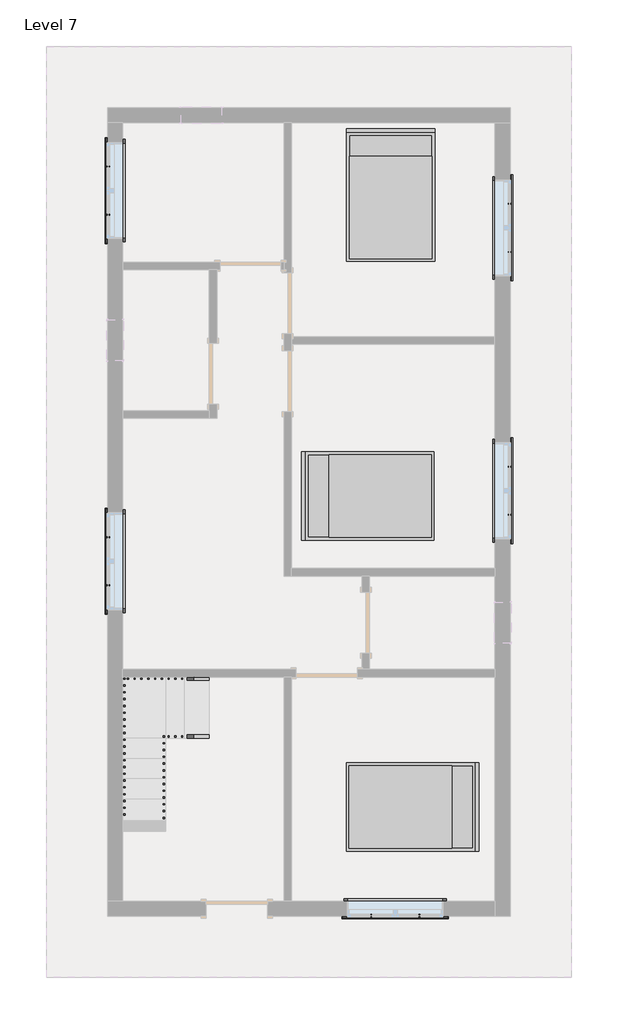
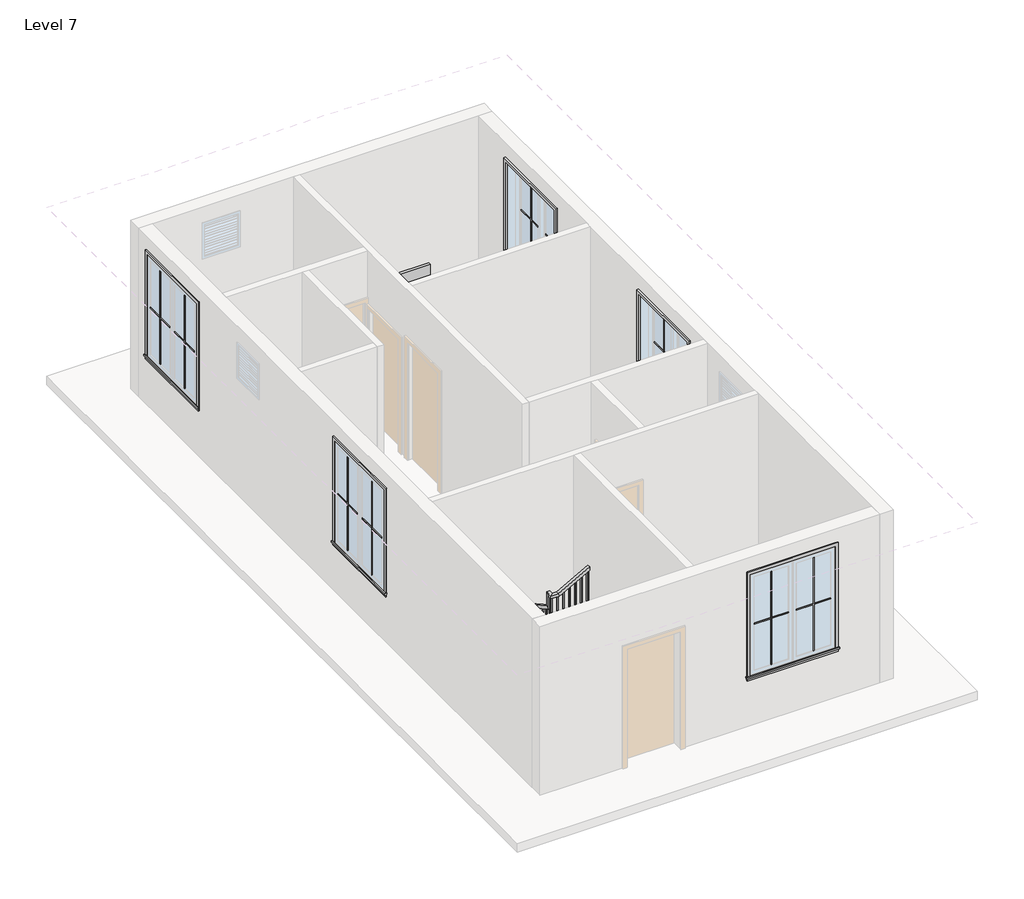
# One storey, part 2 of 2: 20 proxies, 3 furniture elements, 2 railings.
"""IFC4 building model written with IfcOpenShell, lengths in millimetres."""

from ifc_helpers import new_model, si_unit, frame, origin, place, context, project, spatial, polyline, outline, extrude, faceted_brep, transform, mapped, element, save
from components import muntin_pattern_2x2_muntin_pattern_2x2_bff912c5, muntin_pattern_2x2_muntin_pattern_2x2_c2194282, trim_window_exterior_flat_with_sill_e04b3088, trim_window_interior_flat_picture_frame_2a7685fe, bed_17739_bed_17739_15c61121

model = new_model("IFC4")

# Units and contexts
model_context = context("Model", 3, world=origin())
ifc_project = project(units=[si_unit("LENGTHUNIT", "METRE", prefix="MILLI")], contexts=[model_context])

# Site, building, storey
site = spatial("IfcSite", under=ifc_project)
building = spatial("IfcBuilding", under=site)
storey = spatial("IfcBuildingStorey", under=building, Name="Level 7", Elevation=16002.0)

# Proxies
placement = place(None, origin())
muntin_pattern_2x2_muntin_pattern_2x2_shape = muntin_pattern_2x2_muntin_pattern_2x2_bff912c5(model_context)
element("IfcBuildingElementProxy", 1, Name="Muntin Pattern_2x2 : Muntin Pattern_2x2", ObjectType="Muntin Pattern_2x2 : Muntin Pattern_2x2", at=placement, inside=storey, context=model_context, shape_type="MappedRepresentation", body=[
    mapped(muntin_pattern_2x2_muntin_pattern_2x2_shape, transform((-4261.9639285, 4584.2694249, 16986.25), x_axis=(0.0, 1.0, 0.0), y_axis=(-1.0, 0.0, 0.0), z_axis=(0.0, 0.0, 1.0))),
])
element("IfcBuildingElementProxy", 2, Name="Muntin Pattern_2x2 : Muntin Pattern_2x2", ObjectType="Muntin Pattern_2x2 : Muntin Pattern_2x2", at=placement, inside=storey, context=model_context, shape_type="MappedRepresentation", body=[
    mapped(muntin_pattern_2x2_muntin_pattern_2x2_shape, transform((1751.4860715, 4746.1944249, 16986.25), x_axis=(0.0, -1.0, 0.0), y_axis=(1.0, 0.0, 0.0), z_axis=(0.0, 0.0, 1.0))),
])
element("IfcBuildingElementProxy", 3, Name="Muntin Pattern_2x2 : Muntin Pattern_2x2", ObjectType="Muntin Pattern_2x2 : Muntin Pattern_2x2", at=placement, inside=storey, context=model_context, shape_type="MappedRepresentation", body=[
    mapped(muntin_pattern_2x2_muntin_pattern_2x2_shape, transform((-4261.9639285, -962.4555751, 16986.25), x_axis=(0.0, 1.0, 0.0), y_axis=(-1.0, 0.0, 0.0), z_axis=(0.0, 0.0, 1.0))),
])
element("IfcBuildingElementProxy", 4, Name="Muntin Pattern_2x2 : Muntin Pattern_2x2", ObjectType="Muntin Pattern_2x2 : Muntin Pattern_2x2", at=placement, inside=storey, context=model_context, shape_type="MappedRepresentation", body=[
    mapped(muntin_pattern_2x2_muntin_pattern_2x2_shape, transform((1751.4860715, 812.3694249, 16986.25), x_axis=(0.0, -1.0, 0.0), y_axis=(1.0, 0.0, 0.0), z_axis=(0.0, 0.0, 1.0))),
])
element("IfcBuildingElementProxy", 5, Name="Muntin Pattern_2x2 : Muntin Pattern_2x2", ObjectType="Muntin Pattern_2x2 : Muntin Pattern_2x2", at=placement, inside=storey, context=model_context, shape_type="MappedRepresentation", body=[
    mapped(muntin_pattern_2x2_muntin_pattern_2x2_shape, transform((397.3485715, -5907.5180751, 16986.25), x_axis=(-1.0, 0.0, 0.0), y_axis=(0.0, -1.0, 0.0), z_axis=(0.0, 0.0, 1.0))),
])
muntin_pattern_2x2_muntin_pattern_2x2_2_shape = muntin_pattern_2x2_muntin_pattern_2x2_c2194282(model_context)
element("IfcBuildingElementProxy", 6, Name="Muntin Pattern_2x2 : Muntin Pattern_2x2", ObjectType="Muntin Pattern_2x2 : Muntin Pattern_2x2", at=placement, inside=storey, context=model_context, shape_type="MappedRepresentation", body=[
    mapped(muntin_pattern_2x2_muntin_pattern_2x2_2_shape, transform((-4261.9639285, 5304.9944249, 16986.25), x_axis=(0.0, -1.0, 0.0), y_axis=(1.0, 0.0, 0.0), z_axis=(0.0, 0.0, 1.0))),
])
element("IfcBuildingElementProxy", 7, Name="Muntin Pattern_2x2 : Muntin Pattern_2x2", ObjectType="Muntin Pattern_2x2 : Muntin Pattern_2x2", at=placement, inside=storey, context=model_context, shape_type="MappedRepresentation", body=[
    mapped(muntin_pattern_2x2_muntin_pattern_2x2_2_shape, transform((1751.4860715, 4025.4694249, 16986.25), x_axis=(0.0, 1.0, 0.0), y_axis=(-1.0, 0.0, 0.0), z_axis=(0.0, 0.0, 1.0))),
])
element("IfcBuildingElementProxy", 8, Name="Muntin Pattern_2x2 : Muntin Pattern_2x2", ObjectType="Muntin Pattern_2x2 : Muntin Pattern_2x2", at=placement, inside=storey, context=model_context, shape_type="MappedRepresentation", body=[
    mapped(muntin_pattern_2x2_muntin_pattern_2x2_2_shape, transform((-4261.9639285, -241.7305751, 16986.25), x_axis=(0.0, -1.0, 0.0), y_axis=(1.0, 0.0, 0.0), z_axis=(0.0, 0.0, 1.0))),
])
element("IfcBuildingElementProxy", 9, Name="Muntin Pattern_2x2 : Muntin Pattern_2x2", ObjectType="Muntin Pattern_2x2 : Muntin Pattern_2x2", at=placement, inside=storey, context=model_context, shape_type="MappedRepresentation", body=[
    mapped(muntin_pattern_2x2_muntin_pattern_2x2_2_shape, transform((1751.4860715, 91.6444249, 16986.25), x_axis=(0.0, 1.0, 0.0), y_axis=(-1.0, 0.0, 0.0), z_axis=(0.0, 0.0, 1.0))),
])
element("IfcBuildingElementProxy", 10, Name="Muntin Pattern_2x2 : Muntin Pattern_2x2", ObjectType="Muntin Pattern_2x2 : Muntin Pattern_2x2", at=placement, inside=storey, context=model_context, shape_type="MappedRepresentation", body=[
    mapped(muntin_pattern_2x2_muntin_pattern_2x2_2_shape, transform((-323.3764285, -5907.5180751, 16986.25), x_axis=(1.0, 0.0, 0.0), y_axis=(0.0, 1.0, 0.0), z_axis=(0.0, 0.0, 1.0))),
])
trim_window_exterior_flat_with_sill_shape = trim_window_exterior_flat_with_sill_e04b3088(model_context)
element("IfcBuildingElementProxy", 11, Name="Trim-Window-Exterior-Flat : with Sill", ObjectType="Trim-Window-Exterior-Flat : with Sill", at=placement, inside=storey, context=model_context, shape_type="MappedRepresentation", body=[
    mapped(trim_window_exterior_flat_with_sill_shape, transform((-4271.4889285, 4944.6319249, 18745.2), x_axis=(0.0, -1.0, 0.0), y_axis=(0.0, 0.0, 1.0), z_axis=(-1.0, 0.0, 0.0))),
])
element("IfcBuildingElementProxy", 12, Name="Trim-Window-Exterior-Flat : with Sill", ObjectType="Trim-Window-Exterior-Flat : with Sill", at=placement, inside=storey, context=model_context, shape_type="MappedRepresentation", body=[
    mapped(trim_window_exterior_flat_with_sill_shape, transform((1761.0110715, 4385.8319249, 18745.2), x_axis=(0.0, 1.0, 0.0), y_axis=(0.0, 0.0, 1.0), z_axis=(1.0, 0.0, 0.0))),
])
element("IfcBuildingElementProxy", 13, Name="Trim-Window-Exterior-Flat : with Sill", ObjectType="Trim-Window-Exterior-Flat : with Sill", at=placement, inside=storey, context=model_context, shape_type="MappedRepresentation", body=[
    mapped(trim_window_exterior_flat_with_sill_shape, transform((-4271.4889285, -602.0930751, 18745.2), x_axis=(0.0, -1.0, 0.0), y_axis=(0.0, 0.0, 1.0), z_axis=(-1.0, 0.0, 0.0))),
])
element("IfcBuildingElementProxy", 14, Name="Trim-Window-Exterior-Flat : with Sill", ObjectType="Trim-Window-Exterior-Flat : with Sill", at=placement, inside=storey, context=model_context, shape_type="MappedRepresentation", body=[
    mapped(trim_window_exterior_flat_with_sill_shape, transform((1761.0110715, 452.0069249, 18745.2), x_axis=(0.0, 1.0, 0.0), y_axis=(0.0, 0.0, 1.0), z_axis=(1.0, 0.0, 0.0))),
])
element("IfcBuildingElementProxy", 15, Name="Trim-Window-Exterior-Flat : with Sill", ObjectType="Trim-Window-Exterior-Flat : with Sill", at=placement, inside=storey, context=model_context, shape_type="MappedRepresentation", body=[
    mapped(trim_window_exterior_flat_with_sill_shape, transform((36.9860715, -5917.0430751, 18745.2), x_axis=(1.0, 0.0, 0.0), y_axis=(0.0, 0.0, 1.0), z_axis=(0.0, -1.0, 0.0))),
])
trim_window_interior_flat_picture_frame_shape = trim_window_interior_flat_picture_frame_2a7685fe(model_context)
element("IfcBuildingElementProxy", 16, Name="Trim-Window-Interior-Flat : Picture Frame", ObjectType="Trim-Window-Interior-Flat : Picture Frame", at=placement, inside=storey, context=model_context, shape_type="MappedRepresentation", body=[
    mapped(trim_window_interior_flat_picture_frame_shape, transform((-4042.8889285, 4944.6319249, 18745.2), x_axis=(0.0, 1.0, 0.0), y_axis=(0.0, 0.0, 1.0), z_axis=(1.0, 0.0, 0.0))),
])
element("IfcBuildingElementProxy", 17, Name="Trim-Window-Interior-Flat : Picture Frame", ObjectType="Trim-Window-Interior-Flat : Picture Frame", at=placement, inside=storey, context=model_context, shape_type="MappedRepresentation", body=[
    mapped(trim_window_interior_flat_picture_frame_shape, transform((1532.4110715, 4385.8319249, 18745.2), x_axis=(0.0, -1.0, 0.0), y_axis=(0.0, 0.0, 1.0), z_axis=(-1.0, 0.0, 0.0))),
])
element("IfcBuildingElementProxy", 18, Name="Trim-Window-Interior-Flat : Picture Frame", ObjectType="Trim-Window-Interior-Flat : Picture Frame", at=placement, inside=storey, context=model_context, shape_type="MappedRepresentation", body=[
    mapped(trim_window_interior_flat_picture_frame_shape, transform((-4042.8889285, -602.0930751, 18745.2), x_axis=(0.0, 1.0, 0.0), y_axis=(0.0, 0.0, 1.0), z_axis=(1.0, 0.0, 0.0))),
])
element("IfcBuildingElementProxy", 19, Name="Trim-Window-Interior-Flat : Picture Frame", ObjectType="Trim-Window-Interior-Flat : Picture Frame", at=placement, inside=storey, context=model_context, shape_type="MappedRepresentation", body=[
    mapped(trim_window_interior_flat_picture_frame_shape, transform((1532.4110715, 452.0069249, 18745.2), x_axis=(0.0, -1.0, 0.0), y_axis=(0.0, 0.0, 1.0), z_axis=(-1.0, 0.0, 0.0))),
])
element("IfcBuildingElementProxy", 20, Name="Trim-Window-Interior-Flat : Picture Frame", ObjectType="Trim-Window-Interior-Flat : Picture Frame", at=placement, inside=storey, context=model_context, shape_type="MappedRepresentation", body=[
    mapped(trim_window_interior_flat_picture_frame_shape, transform((36.9860715, -5688.4430751, 18745.2), x_axis=(-1.0, 0.0, 0.0), y_axis=(0.0, 0.0, 1.0), z_axis=(0.0, 1.0, 0.0))),
])

# Furniture
bed_17739_bed_17739_shape = bed_17739_bed_17739_15c61121(model_context)
element("IfcFurniture", 21, ObjectType="Bed_17739 : Bed_17739", at=placement, inside=storey, context=model_context, shape_type="MappedRepresentation", body=[
    mapped(bed_17739_bed_17739_shape, transform((-29.6889285, 4852.5569249, 16002.0), x_axis=(1.0, 0.0, 0.0), y_axis=(0.0, 1.0, 0.0), z_axis=(0.0, 0.0, 1.0))),
])
element("IfcFurniture", 22, ObjectType="Bed_17739 : Bed_17739", at=placement, inside=storey, context=model_context, shape_type="MappedRepresentation", body=[
    mapped(bed_17739_bed_17739_shape, transform((-347.1889285, 375.8069249, 16002.0), x_axis=(0.0, 1.0, 0.0), y_axis=(-1.0, 0.0, 0.0), z_axis=(0.0, 0.0, 1.0))),
])
element("IfcFurniture", 23, ObjectType="Bed_17739 : Bed_17739", at=placement, inside=storey, context=model_context, shape_type="MappedRepresentation", body=[
    mapped(bed_17739_bed_17739_shape, transform((275.1110715, -4278.7430751, 16002.0), x_axis=(0.0, -1.0, 0.0), y_axis=(1.0, 0.0, 0.0), z_axis=(0.0, 0.0, 1.0))),
])

# Railings
element("IfcRailing", 24, ObjectType="Handrail - Rectangular", at=placement, inside=storey, context=model_context, shape_type="SolidModel", body=[
    faceted_brep([(-2747.4889285, -2386.4430751, 17085.7333333), (-2747.4889285, -2386.4430751, 17028.5271159), (-2747.4889285, -2335.6430751, 17028.5271159), (-2747.4889285, -2335.6430751, 17085.7333333), (-3396.0267484, -2386.4430751, 17421.5457967), (-3408.3987558, -2386.4430751, 17370.7457967), (-3408.3987558, -2335.6430751, 17370.7457967), (-3396.0267484, -2335.6430751, 17421.5457967), (-3992.0889285, -2386.4430751, 17421.5457967), (-3992.0889285, -2386.4430751, 17370.7457967), (-4042.8889285, -2335.6430751, 17370.7457967), (-4042.8889285, -2335.6430751, 17421.5457967), (-3992.0889285, -2940.1628326, 17421.5457967), (-3992.0889285, -2953.3285634, 17370.7457967), (-4042.8889285, -2953.3285634, 17370.7457967), (-4042.8889285, -2940.1628326, 17421.5457967), (-3992.0889285, -5061.9991591, 18600.5618165), (-3992.0889285, -5075.1648899, 18549.7618165), (-4042.8889285, -5075.1648899, 18549.7618165), (-4042.8889285, -5061.9991591, 18600.5618165), (-3992.0889285, -5637.6430751, 18600.5618165), (-3992.0889285, -5637.6430751, 18549.7618165), (-4042.8889285, -5688.4430751, 18549.7618165), (-4042.8889285, -5688.4430751, 18600.5618165), (-3418.001852, -5637.6430751, 18600.5618165), (-3404.8062484, -5637.6430751, 18549.7618165), (-3404.8062484, -5688.4430751, 18549.7618165), (-3418.001852, -5688.4430751, 18600.5618165), (-2793.6303845, -5637.6430751, 18948.4), (-2793.6303845, -5688.4430751, 18948.4), (-2793.6303845, -5688.4430751, 18890.2487115), (-2793.6303845, -5637.6430751, 18890.2487115)], [[[0, 1, 2, 3]], [[1, 0, 4, 5]], [[2, 1, 5, 6]], [[3, 2, 6, 7]], [[0, 3, 7, 4]], [[5, 4, 8, 9]], [[6, 5, 9, 10]], [[7, 6, 10, 11]], [[4, 7, 11, 8]], [[9, 8, 12, 13]], [[10, 9, 13, 14]], [[11, 10, 14, 15]], [[8, 11, 15, 12]], [[13, 12, 16, 17]], [[14, 13, 17, 18]], [[15, 14, 18, 19]], [[12, 15, 19, 16]], [[17, 16, 20, 21]], [[18, 17, 21, 22]], [[19, 18, 22, 23]], [[16, 19, 23, 20]], [[21, 20, 24, 25]], [[22, 21, 25, 26]], [[23, 22, 26, 27]], [[20, 23, 27, 24]], [[28, 29, 30, 31]], [[25, 24, 28, 31]], [[26, 25, 31, 30]], [[27, 26, 30, 29]], [[24, 27, 29, 28]]]),
    extrude(outline(polyline([(18892.9598207, -2788.7639285), (18882.3470401, -2807.8139285), (17864.6666667, -2807.8139285), (17864.6666667, -2788.7639285), (18892.9598207, -2788.7639285)])), frame((0.0, -5672.5680751, 0.0), z_axis=(0.0, 1.0, 0.0), x_axis=(0.0, 0.0, 1.0)), (0.0, 0.0, 1.0), 19.05),
    extrude(outline(polyline([(18836.3583242, -2890.3639285), (18825.7455436, -2909.4139285), (17864.6666667, -2909.4139285), (17864.6666667, -2890.3639285), (18836.3583242, -2890.3639285)])), frame((0.0, -5672.5680751, 0.0), z_axis=(0.0, 1.0, 0.0), x_axis=(0.0, 0.0, 1.0)), (0.0, 0.0, 1.0), 19.05),
    extrude(outline(polyline([(18779.7568277, -2991.9639285), (18769.1440471, -3011.0139285), (17864.6666667, -3011.0139285), (17864.6666667, -2991.9639285), (18779.7568277, -2991.9639285)])), frame((0.0, -5672.5680751, 0.0), z_axis=(0.0, 1.0, 0.0), x_axis=(0.0, 0.0, 1.0)), (0.0, 0.0, 1.0), 19.05),
    extrude(outline(polyline([(18723.1553312, -3093.5639285), (18712.5425506, -3112.6139285), (17864.6666667, -3112.6139285), (17864.6666667, -3093.5639285), (18723.1553312, -3093.5639285)])), frame((0.0, -5672.5680751, 0.0), z_axis=(0.0, 1.0, 0.0), x_axis=(0.0, 0.0, 1.0)), (0.0, 0.0, 1.0), 19.05),
    extrude(outline(polyline([(18666.5538346, -3195.1639285), (18655.9410541, -3214.2139285), (17695.3333333, -3214.2139285), (17695.3333333, -3195.1639285), (18666.5538346, -3195.1639285)])), frame((0.0, -5672.5680751, 0.0), z_axis=(0.0, 1.0, 0.0), x_axis=(0.0, 0.0, 1.0)), (0.0, 0.0, 1.0), 19.05),
    extrude(outline(polyline([(18609.9523381, -3296.7639285), (18599.3395575, -3315.8139285), (17695.3333333, -3315.8139285), (17695.3333333, -3296.7639285), (18609.9523381, -3296.7639285)])), frame((0.0, -5672.5680751, 0.0), z_axis=(0.0, 1.0, 0.0), x_axis=(0.0, 0.0, 1.0)), (0.0, 0.0, 1.0), 19.05),
    extrude(outline(polyline([(18553.3508416, -3398.3639285), (18542.738061, -3417.4139285), (17526.0, -3417.4139285), (17526.0, -3398.3639285), (18553.3508416, -3398.3639285)])), frame((0.0, -5672.5680751, 0.0), z_axis=(0.0, 1.0, 0.0), x_axis=(0.0, 0.0, 1.0)), (0.0, 0.0, 1.0), 19.05),
    extrude(outline(polyline([(-3519.0139285, -5672.5680751), (-3519.0139285, -5653.5180751), (-3499.9639285, -5653.5180751), (-3499.9639285, -5672.5680751), (-3519.0139285, -5672.5680751)])), frame((0.0, 0.0, 17526.0), z_axis=(0.0, 0.0, 1.0), x_axis=(1.0, 0.0, 0.0)), (0.0, 0.0, 1.0), 1023.7618165),
    extrude(outline(polyline([(-3620.6139285, -5672.5680751), (-3620.6139285, -5653.5180751), (-3601.5639285, -5653.5180751), (-3601.5639285, -5672.5680751), (-3620.6139285, -5672.5680751)])), frame((0.0, 0.0, 17526.0), z_axis=(0.0, 0.0, 1.0), x_axis=(1.0, 0.0, 0.0)), (0.0, 0.0, 1.0), 1023.7618165),
    extrude(outline(polyline([(-3722.2139285, -5672.5680751), (-3722.2139285, -5653.5180751), (-3703.1639285, -5653.5180751), (-3703.1639285, -5672.5680751), (-3722.2139285, -5672.5680751)])), frame((0.0, 0.0, 17526.0), z_axis=(0.0, 0.0, 1.0), x_axis=(1.0, 0.0, 0.0)), (0.0, 0.0, 1.0), 1023.7618165),
    extrude(outline(polyline([(-3823.8139285, -5672.5680751), (-3823.8139285, -5653.5180751), (-3804.7639285, -5653.5180751), (-3804.7639285, -5672.5680751), (-3823.8139285, -5672.5680751)])), frame((0.0, 0.0, 17526.0), z_axis=(0.0, 0.0, 1.0), x_axis=(1.0, 0.0, 0.0)), (0.0, 0.0, 1.0), 1023.7618165),
    extrude(outline(polyline([(-3925.4139285, -5672.5680751), (-3925.4139285, -5653.5180751), (-3906.3639285, -5653.5180751), (-3906.3639285, -5672.5680751), (-3925.4139285, -5672.5680751)])), frame((0.0, 0.0, 17526.0), z_axis=(0.0, 0.0, 1.0), x_axis=(1.0, 0.0, 0.0)), (0.0, 0.0, 1.0), 1023.7618165),
    extrude(outline(polyline([(-4027.0139285, -5602.7180751), (-4007.9639285, -5602.7180751), (-4007.9639285, -5621.7680751), (-4027.0139285, -5621.7680751), (-4027.0139285, -5602.7180751)])), frame((0.0, 0.0, 17526.0), z_axis=(0.0, 0.0, 1.0), x_axis=(1.0, 0.0, 0.0)), (0.0, 0.0, 1.0), 1023.7618165),
    extrude(outline(polyline([(-4027.0139285, -5501.1180751), (-4007.9639285, -5501.1180751), (-4007.9639285, -5520.1680751), (-4027.0139285, -5520.1680751), (-4027.0139285, -5501.1180751)])), frame((0.0, 0.0, 17526.0), z_axis=(0.0, 0.0, 1.0), x_axis=(1.0, 0.0, 0.0)), (0.0, 0.0, 1.0), 1023.7618165),
    extrude(outline(polyline([(-4027.0139285, -5399.5180751), (-4007.9639285, -5399.5180751), (-4007.9639285, -5418.5680751), (-4027.0139285, -5418.5680751), (-4027.0139285, -5399.5180751)])), frame((0.0, 0.0, 17526.0), z_axis=(0.0, 0.0, 1.0), x_axis=(1.0, 0.0, 0.0)), (0.0, 0.0, 1.0), 1023.7618165),
    extrude(outline(polyline([(-4027.0139285, -5297.9180751), (-4007.9639285, -5297.9180751), (-4007.9639285, -5316.9680751), (-4027.0139285, -5316.9680751), (-4027.0139285, -5297.9180751)])), frame((0.0, 0.0, 17526.0), z_axis=(0.0, 0.0, 1.0), x_axis=(1.0, 0.0, 0.0)), (0.0, 0.0, 1.0), 1023.7618165),
    extrude(outline(polyline([(-4027.0139285, -5196.3180751), (-4007.9639285, -5196.3180751), (-4007.9639285, -5215.3680751), (-4027.0139285, -5215.3680751), (-4027.0139285, -5196.3180751)])), frame((0.0, 0.0, 17526.0), z_axis=(0.0, 0.0, 1.0), x_axis=(1.0, 0.0, 0.0)), (0.0, 0.0, 1.0), 1023.7618165),
    extrude(outline(polyline([(-4027.0139285, -5094.7180751), (-4007.9639285, -5094.7180751), (-4007.9639285, -5113.7680751), (-4027.0139285, -5113.7680751), (-4027.0139285, -5094.7180751)])), frame((0.0, 0.0, 17526.0), z_axis=(0.0, 0.0, 1.0), x_axis=(1.0, 0.0, 0.0)), (0.0, 0.0, 1.0), 1023.7618165),
    extrude(outline(polyline([(-5012.1680751, 18514.7571119), (-4993.1180751, 18504.1718208), (-4993.1180751, 17526.0), (-5012.1680751, 17526.0), (-5012.1680751, 18514.7571119)])), frame((-4027.0139285, 0.0, 0.0), z_axis=(1.0, 0.0, 0.0), x_axis=(0.0, 1.0, 0.0)), (0.0, 0.0, 1.0), 19.05),
    extrude(outline(polyline([(-4910.5680751, 18458.3022261), (-4891.5180751, 18447.716935), (-4891.5180751, 17526.0), (-4910.5680751, 17526.0), (-4910.5680751, 18458.3022261)])), frame((-4027.0139285, 0.0, 0.0), z_axis=(1.0, 0.0, 0.0), x_axis=(0.0, 1.0, 0.0)), (0.0, 0.0, 1.0), 19.05),
    extrude(outline(polyline([(-4808.9680751, 18401.8473402), (-4789.9180751, 18391.2620491), (-4789.9180751, 17526.0), (-4808.9680751, 17526.0), (-4808.9680751, 18401.8473402)])), frame((-4027.0139285, 0.0, 0.0), z_axis=(1.0, 0.0, 0.0), x_axis=(0.0, 1.0, 0.0)), (0.0, 0.0, 1.0), 19.05),
    extrude(outline(polyline([(-4707.3680751, 18345.2358332), (-4688.3180751, 18334.6505421), (-4688.3180751, 17356.6666667), (-4707.3680751, 17356.6666667), (-4707.3680751, 18345.2358332)])), frame((-4027.0139285, 0.0, 0.0), z_axis=(1.0, 0.0, 0.0), x_axis=(0.0, 1.0, 0.0)), (0.0, 0.0, 1.0), 19.05),
    extrude(outline(polyline([(-4605.7680751, 18288.7809474), (-4586.7180751, 18278.1956563), (-4586.7180751, 17356.6666667), (-4605.7680751, 17356.6666667), (-4605.7680751, 18288.7809474)])), frame((-4027.0139285, 0.0, 0.0), z_axis=(1.0, 0.0, 0.0), x_axis=(0.0, 1.0, 0.0)), (0.0, 0.0, 1.0), 19.05),
    extrude(outline(polyline([(-4504.1680751, 18232.3260615), (-4485.1180751, 18221.7407704), (-4485.1180751, 17356.6666667), (-4504.1680751, 17356.6666667), (-4504.1680751, 18232.3260615)])), frame((-4027.0139285, 0.0, 0.0), z_axis=(1.0, 0.0, 0.0), x_axis=(0.0, 1.0, 0.0)), (0.0, 0.0, 1.0), 19.05),
    extrude(outline(polyline([(-4402.5680751, 18175.9024999), (-4383.5180751, 18165.3172088), (-4383.5180751, 17187.3333333), (-4402.5680751, 17187.3333333), (-4402.5680751, 18175.9024999)])), frame((-4027.0139285, 0.0, 0.0), z_axis=(1.0, 0.0, 0.0), x_axis=(0.0, 1.0, 0.0)), (0.0, 0.0, 1.0), 19.05),
    extrude(outline(polyline([(-4300.9680751, 18119.447614), (-4281.9180751, 18108.8623229), (-4281.9180751, 17187.3333333), (-4300.9680751, 17187.3333333), (-4300.9680751, 18119.447614)])), frame((-4027.0139285, 0.0, 0.0), z_axis=(1.0, 0.0, 0.0), x_axis=(0.0, 1.0, 0.0)), (0.0, 0.0, 1.0), 19.05),
    extrude(outline(polyline([(-4199.3680751, 18062.9927282), (-4180.3180751, 18052.4074371), (-4180.3180751, 17187.3333333), (-4199.3680751, 17187.3333333), (-4199.3680751, 18062.9927282)])), frame((-4027.0139285, 0.0, 0.0), z_axis=(1.0, 0.0, 0.0), x_axis=(0.0, 1.0, 0.0)), (0.0, 0.0, 1.0), 19.05),
    extrude(outline(polyline([(-4097.7680751, 18006.5691666), (-4078.7180751, 17995.9838755), (-4078.7180751, 17018.0), (-4097.7680751, 17018.0), (-4097.7680751, 18006.5691666)])), frame((-4027.0139285, 0.0, 0.0), z_axis=(1.0, 0.0, 0.0), x_axis=(0.0, 1.0, 0.0)), (0.0, 0.0, 1.0), 19.05),
    extrude(outline(polyline([(-3996.1680751, 17950.1142807), (-3977.1180751, 17939.5289896), (-3977.1180751, 17018.0), (-3996.1680751, 17018.0), (-3996.1680751, 17950.1142807)])), frame((-4027.0139285, 0.0, 0.0), z_axis=(1.0, 0.0, 0.0), x_axis=(0.0, 1.0, 0.0)), (0.0, 0.0, 1.0), 19.05),
    extrude(outline(polyline([(-3894.5680751, 17893.6593949), (-3875.5180751, 17883.0741038), (-3875.5180751, 17018.0), (-3894.5680751, 17018.0), (-3894.5680751, 17893.6593949)])), frame((-4027.0139285, 0.0, 0.0), z_axis=(1.0, 0.0, 0.0), x_axis=(0.0, 1.0, 0.0)), (0.0, 0.0, 1.0), 19.05),
    extrude(outline(polyline([(-3792.9680751, 17837.2358332), (-3773.9180751, 17826.6505421), (-3773.9180751, 16848.6666667), (-3792.9680751, 16848.6666667), (-3792.9680751, 17837.2358332)])), frame((-4027.0139285, 0.0, 0.0), z_axis=(1.0, 0.0, 0.0), x_axis=(0.0, 1.0, 0.0)), (0.0, 0.0, 1.0), 19.05),
    extrude(outline(polyline([(-3691.3680751, 17780.7809474), (-3672.3180751, 17770.1956563), (-3672.3180751, 16848.6666667), (-3691.3680751, 16848.6666667), (-3691.3680751, 17780.7809474)])), frame((-4027.0139285, 0.0, 0.0), z_axis=(1.0, 0.0, 0.0), x_axis=(0.0, 1.0, 0.0)), (0.0, 0.0, 1.0), 19.05),
    extrude(outline(polyline([(-3589.7680751, 17724.3260615), (-3570.7180751, 17713.7407704), (-3570.7180751, 16848.6666667), (-3589.7680751, 16848.6666667), (-3589.7680751, 17724.3260615)])), frame((-4027.0139285, 0.0, 0.0), z_axis=(1.0, 0.0, 0.0), x_axis=(0.0, 1.0, 0.0)), (0.0, 0.0, 1.0), 19.05),
    extrude(outline(polyline([(-3488.1680751, 17667.9024999), (-3469.1180751, 17657.3172088), (-3469.1180751, 16679.3333333), (-3488.1680751, 16679.3333333), (-3488.1680751, 17667.9024999)])), frame((-4027.0139285, 0.0, 0.0), z_axis=(1.0, 0.0, 0.0), x_axis=(0.0, 1.0, 0.0)), (0.0, 0.0, 1.0), 19.05),
    extrude(outline(polyline([(-3386.5680751, 17611.447614), (-3367.5180751, 17600.8623229), (-3367.5180751, 16679.3333333), (-3386.5680751, 16679.3333333), (-3386.5680751, 17611.447614)])), frame((-4027.0139285, 0.0, 0.0), z_axis=(1.0, 0.0, 0.0), x_axis=(0.0, 1.0, 0.0)), (0.0, 0.0, 1.0), 19.05),
    extrude(outline(polyline([(-3284.9680751, 17554.9927282), (-3265.9180751, 17544.4074371), (-3265.9180751, 16679.3333333), (-3284.9680751, 16679.3333333), (-3284.9680751, 17554.9927282)])), frame((-4027.0139285, 0.0, 0.0), z_axis=(1.0, 0.0, 0.0), x_axis=(0.0, 1.0, 0.0)), (0.0, 0.0, 1.0), 19.05),
    extrude(outline(polyline([(-3183.3680751, 17498.5691666), (-3164.3180751, 17487.9838755), (-3164.3180751, 16510.0), (-3183.3680751, 16510.0), (-3183.3680751, 17498.5691666)])), frame((-4027.0139285, 0.0, 0.0), z_axis=(1.0, 0.0, 0.0), x_axis=(0.0, 1.0, 0.0)), (0.0, 0.0, 1.0), 19.05),
    extrude(outline(polyline([(-3081.7680751, 17442.1142807), (-3062.7180751, 17431.5289896), (-3062.7180751, 16510.0), (-3081.7680751, 16510.0), (-3081.7680751, 17442.1142807)])), frame((-4027.0139285, 0.0, 0.0), z_axis=(1.0, 0.0, 0.0), x_axis=(0.0, 1.0, 0.0)), (0.0, 0.0, 1.0), 19.05),
    extrude(outline(polyline([(-2980.1680751, 17385.6593949), (-2961.1180751, 17375.0741038), (-2961.1180751, 16510.0), (-2980.1680751, 16510.0), (-2980.1680751, 17385.6593949)])), frame((-4027.0139285, 0.0, 0.0), z_axis=(1.0, 0.0, 0.0), x_axis=(0.0, 1.0, 0.0)), (0.0, 0.0, 1.0), 19.05),
    extrude(outline(polyline([(-4027.0139285, -2859.5180751), (-4007.9639285, -2859.5180751), (-4007.9639285, -2878.5680751), (-4027.0139285, -2878.5680751), (-4027.0139285, -2859.5180751)])), frame((0.0, 0.0, 16510.0), z_axis=(0.0, 0.0, 1.0), x_axis=(1.0, 0.0, 0.0)), (0.0, 0.0, 1.0), 860.7457967),
    extrude(outline(polyline([(-4027.0139285, -2757.9180751), (-4007.9639285, -2757.9180751), (-4007.9639285, -2776.9680751), (-4027.0139285, -2776.9680751), (-4027.0139285, -2757.9180751)])), frame((0.0, 0.0, 16510.0), z_axis=(0.0, 0.0, 1.0), x_axis=(1.0, 0.0, 0.0)), (0.0, 0.0, 1.0), 860.7457967),
    extrude(outline(polyline([(-4027.0139285, -2656.3180751), (-4007.9639285, -2656.3180751), (-4007.9639285, -2675.3680751), (-4027.0139285, -2675.3680751), (-4027.0139285, -2656.3180751)])), frame((0.0, 0.0, 16510.0), z_axis=(0.0, 0.0, 1.0), x_axis=(1.0, 0.0, 0.0)), (0.0, 0.0, 1.0), 860.7457967),
    extrude(outline(polyline([(-4027.0139285, -2554.7180751), (-4007.9639285, -2554.7180751), (-4007.9639285, -2573.7680751), (-4027.0139285, -2573.7680751), (-4027.0139285, -2554.7180751)])), frame((0.0, 0.0, 16510.0), z_axis=(0.0, 0.0, 1.0), x_axis=(1.0, 0.0, 0.0)), (0.0, 0.0, 1.0), 860.7457967),
    extrude(outline(polyline([(-4027.0139285, -2453.1180751), (-4007.9639285, -2453.1180751), (-4007.9639285, -2472.1680751), (-4027.0139285, -2472.1680751), (-4027.0139285, -2453.1180751)])), frame((0.0, 0.0, 16510.0), z_axis=(0.0, 0.0, 1.0), x_axis=(1.0, 0.0, 0.0)), (0.0, 0.0, 1.0), 860.7457967),
    extrude(outline(polyline([(-3957.1639285, -2351.5180751), (-3957.1639285, -2370.5680751), (-3976.2139285, -2370.5680751), (-3976.2139285, -2351.5180751), (-3957.1639285, -2351.5180751)])), frame((0.0, 0.0, 16510.0), z_axis=(0.0, 0.0, 1.0), x_axis=(1.0, 0.0, 0.0)), (0.0, 0.0, 1.0), 860.7457967),
    extrude(outline(polyline([(-3855.5639285, -2351.5180751), (-3855.5639285, -2370.5680751), (-3874.6139285, -2370.5680751), (-3874.6139285, -2351.5180751), (-3855.5639285, -2351.5180751)])), frame((0.0, 0.0, 16510.0), z_axis=(0.0, 0.0, 1.0), x_axis=(1.0, 0.0, 0.0)), (0.0, 0.0, 1.0), 860.7457967),
    extrude(outline(polyline([(-3753.9639285, -2351.5180751), (-3753.9639285, -2370.5680751), (-3773.0139285, -2370.5680751), (-3773.0139285, -2351.5180751), (-3753.9639285, -2351.5180751)])), frame((0.0, 0.0, 16510.0), z_axis=(0.0, 0.0, 1.0), x_axis=(1.0, 0.0, 0.0)), (0.0, 0.0, 1.0), 860.7457967),
    extrude(outline(polyline([(-3652.3639285, -2351.5180751), (-3652.3639285, -2370.5680751), (-3671.4139285, -2370.5680751), (-3671.4139285, -2351.5180751), (-3652.3639285, -2351.5180751)])), frame((0.0, 0.0, 16510.0), z_axis=(0.0, 0.0, 1.0), x_axis=(1.0, 0.0, 0.0)), (0.0, 0.0, 1.0), 860.7457967),
    extrude(outline(polyline([(-3550.7639285, -2351.5180751), (-3550.7639285, -2370.5680751), (-3569.8139285, -2370.5680751), (-3569.8139285, -2351.5180751), (-3550.7639285, -2351.5180751)])), frame((0.0, 0.0, 16510.0), z_axis=(0.0, 0.0, 1.0), x_axis=(1.0, 0.0, 0.0)), (0.0, 0.0, 1.0), 860.7457967),
    extrude(outline(polyline([(-3449.1639285, -2351.5180751), (-3449.1639285, -2370.5680751), (-3468.2139285, -2370.5680751), (-3468.2139285, -2351.5180751), (-3449.1639285, -2351.5180751)])), frame((0.0, 0.0, 16510.0), z_axis=(0.0, 0.0, 1.0), x_axis=(1.0, 0.0, 0.0)), (0.0, 0.0, 1.0), 860.7457967),
    extrude(outline(polyline([(17339.2455625, -3347.5639285), (17349.1096402, -3366.6139285), (16340.6666667, -3366.6139285), (16340.6666667, -3347.5639285), (17339.2455625, -3347.5639285)])), frame((0.0, -2370.5680751, 0.0), z_axis=(0.0, 1.0, 0.0), x_axis=(0.0, 0.0, 1.0)), (0.0, 0.0, 1.0), 19.05),
    extrude(outline(polyline([(17286.6371483, -3245.9639285), (17296.5012259, -3265.0139285), (16340.6666667, -3265.0139285), (16340.6666667, -3245.9639285), (17286.6371483, -3245.9639285)])), frame((0.0, -2370.5680751, 0.0), z_axis=(0.0, 1.0, 0.0), x_axis=(0.0, 0.0, 1.0)), (0.0, 0.0, 1.0), 19.05),
    extrude(outline(polyline([(17234.028734, -3144.3639285), (17243.8928117, -3163.4139285), (16340.6666667, -3163.4139285), (16340.6666667, -3144.3639285), (17234.028734, -3144.3639285)])), frame((0.0, -2370.5680751, 0.0), z_axis=(0.0, 1.0, 0.0), x_axis=(0.0, 0.0, 1.0)), (0.0, 0.0, 1.0), 19.05),
    extrude(outline(polyline([(17181.4203198, -3042.7639285), (17191.2843975, -3061.8139285), (16171.3333333, -3061.8139285), (16171.3333333, -3042.7639285), (17181.4203198, -3042.7639285)])), frame((0.0, -2370.5680751, 0.0), z_axis=(0.0, 1.0, 0.0), x_axis=(0.0, 0.0, 1.0)), (0.0, 0.0, 1.0), 19.05),
    extrude(outline(polyline([(17128.8119056, -2941.1639285), (17138.6759832, -2960.2139285), (16171.3333333, -2960.2139285), (16171.3333333, -2941.1639285), (17128.8119056, -2941.1639285)])), frame((0.0, -2370.5680751, 0.0), z_axis=(0.0, 1.0, 0.0), x_axis=(0.0, 0.0, 1.0)), (0.0, 0.0, 1.0), 19.05),
    extrude(outline(polyline([(17076.2034913, -2839.5639285), (17086.067569, -2858.6139285), (16171.3333333, -2858.6139285), (16171.3333333, -2839.5639285), (17076.2034913, -2839.5639285)])), frame((0.0, -2370.5680751, 0.0), z_axis=(0.0, 1.0, 0.0), x_axis=(0.0, 0.0, 1.0)), (0.0, 0.0, 1.0), 19.05),
    extrude(outline(polyline([(-4027.0139285, -5653.5180751), (-4007.9639285, -5653.5180751), (-4007.9639285, -5672.5680751), (-4027.0139285, -5672.5680751), (-4027.0139285, -5653.5180751)])), frame((0.0, 0.0, 17526.0), z_axis=(0.0, 0.0, 1.0), x_axis=(1.0, 0.0, 0.0)), (0.0, 0.0, 1.0), 1023.7618165),
    extrude(outline(polyline([(-4007.9639285, -2351.5180751), (-4007.9639285, -2370.5680751), (-4027.0139285, -2370.5680751), (-4027.0139285, -2351.5180751), (-4007.9639285, -2351.5180751)])), frame((0.0, 0.0, 16510.0), z_axis=(0.0, 0.0, 1.0), x_axis=(1.0, 0.0, 0.0)), (0.0, 0.0, 1.0), 860.7457967),
    extrude(outline(polyline([(18890.2487115, -2793.6303845), (18879.6359309, -2812.6803845), (17864.6666667, -2812.6803845), (17864.6666667, -2793.6303845), (18890.2487115, -2793.6303845)])), frame((0.0, -5672.5680751, 0.0), z_axis=(0.0, 1.0, 0.0), x_axis=(0.0, 0.0, 1.0)), (0.0, 0.0, 1.0), 19.05),
    extrude(outline(polyline([(17028.5271159, -2747.4889285), (17038.3911936, -2766.5389285), (16171.3333333, -2766.5389285), (16171.3333333, -2747.4889285), (17028.5271159, -2747.4889285)])), frame((0.0, -2370.5680751, 0.0), z_axis=(0.0, 1.0, 0.0), x_axis=(0.0, 0.0, 1.0)), (0.0, 0.0, 1.0), 19.05),
])
element("IfcRailing", 25, ObjectType="Handrail - Rectangular", at=placement, inside=storey, context=model_context, shape_type="SolidModel", body=[
    faceted_brep([(-2747.4889285, -3250.0430751, 17085.7333333), (-2747.4889285, -3250.0430751, 17028.5271159), (-2747.4889285, -3199.2430751, 17028.5271159), (-2747.4889285, -3199.2430751, 17085.7333333), (-3325.3389285, -3250.0430751, 17384.9436893), (-3376.1389285, -3250.0430751, 17354.041679), (-3376.1389285, -3199.2430751, 17354.041679), (-3325.3389285, -3199.2430751, 17384.9436893), (-3325.3389285, -3250.0430751, 17636.0744977), (-3376.1389285, -3250.0430751, 17585.2744977), (-3376.1389285, -3199.2430751, 17585.2744977), (-3325.3389285, -3199.2430751, 17636.0744977), (-3401.5389285, -3250.0430751, 17636.0744977), (-3401.5389285, -3250.0430751, 17585.2744977), (-3452.3389285, -3199.2430751, 17585.2744977), (-3452.3389285, -3199.2430751, 17636.0744977), (-3401.5389285, -3326.2430751, 17636.0744977), (-3401.5389285, -3339.4088059, 17585.2744977), (-3452.3389285, -3339.4088059, 17585.2744977), (-3452.3389285, -3326.2430751, 17636.0744977), (-3401.5389285, -4697.5612092, 18398.0588356), (-3401.5389285, -4748.3612092, 18368.1706306), (-3452.3389285, -4748.3612092, 18368.1706306), (-3452.3389285, -4697.5612092, 18398.0588356), (-3401.5389285, -4697.5612092, 18652.1844557), (-3401.5389285, -4748.3612092, 18601.3844557), (-3452.3389285, -4748.3612092, 18601.3844557), (-3452.3389285, -4697.5612092, 18652.1844557), (-3401.5389285, -4773.7612092, 18652.1844557), (-3401.5389285, -4773.7612092, 18601.3844557), (-3452.3389285, -4824.5612092, 18601.3844557), (-3452.3389285, -4824.5612092, 18652.1844557), (-3325.3389285, -4773.7612092, 18652.1844557), (-3312.1433249, -4773.7612092, 18601.3844557), (-3312.1433249, -4824.5612092, 18601.3844557), (-3325.3389285, -4824.5612092, 18652.1844557), (-2793.6303845, -4773.7612092, 18948.4), (-2793.6303845, -4824.5612092, 18948.4), (-2793.6303845, -4824.5612092, 18890.2487115), (-2793.6303845, -4773.7612092, 18890.2487115)], [[[0, 1, 2, 3]], [[1, 0, 4, 5]], [[2, 1, 5, 6]], [[3, 2, 6, 7]], [[0, 3, 7, 4]], [[5, 4, 8, 9]], [[6, 5, 9, 10]], [[7, 6, 10, 11]], [[4, 7, 11, 8]], [[9, 8, 12, 13]], [[10, 9, 13, 14]], [[11, 10, 14, 15]], [[8, 11, 15, 12]], [[13, 12, 16, 17]], [[14, 13, 17, 18]], [[15, 14, 18, 19]], [[12, 15, 19, 16]], [[17, 16, 20, 21]], [[18, 17, 21, 22]], [[19, 18, 22, 23]], [[16, 19, 23, 20]], [[21, 20, 24, 25]], [[22, 21, 25, 26]], [[23, 22, 26, 27]], [[20, 23, 27, 24]], [[25, 24, 28, 29]], [[26, 25, 29, 30]], [[27, 26, 30, 31]], [[24, 27, 31, 28]], [[29, 28, 32, 33]], [[30, 29, 33, 34]], [[31, 30, 34, 35]], [[28, 31, 35, 32]], [[36, 37, 38, 39]], [[33, 32, 36, 39]], [[34, 33, 39, 38]], [[35, 34, 38, 37]], [[32, 35, 37, 36]]]),
    extrude(outline(polyline([(18871.7342595, -2826.8639285), (17864.6666667, -2826.8639285), (17864.6666667, -2807.8139285), (18882.3470401, -2807.8139285), (18871.7342595, -2826.8639285)])), frame((0.0, -4808.6862092, 0.0), z_axis=(0.0, 1.0, 0.0), x_axis=(0.0, 0.0, 1.0)), (0.0, 0.0, 1.0), 19.05),
    extrude(outline(polyline([(18815.132763, -2928.4639285), (17864.6666667, -2928.4639285), (17864.6666667, -2909.4139285), (18825.7455436, -2909.4139285), (18815.132763, -2928.4639285)])), frame((0.0, -4808.6862092, 0.0), z_axis=(0.0, 1.0, 0.0), x_axis=(0.0, 0.0, 1.0)), (0.0, 0.0, 1.0), 19.05),
    extrude(outline(polyline([(18758.5312665, -3030.0639285), (17864.6666667, -3030.0639285), (17864.6666667, -3011.0139285), (18769.1440471, -3011.0139285), (18758.5312665, -3030.0639285)])), frame((0.0, -4808.6862092, 0.0), z_axis=(0.0, 1.0, 0.0), x_axis=(0.0, 0.0, 1.0)), (0.0, 0.0, 1.0), 19.05),
    extrude(outline(polyline([(18701.92977, -3131.6639285), (17864.6666667, -3131.6639285), (17864.6666667, -3112.6139285), (18712.5425506, -3112.6139285), (18701.92977, -3131.6639285)])), frame((0.0, -4808.6862092, 0.0), z_axis=(0.0, 1.0, 0.0), x_axis=(0.0, 0.0, 1.0)), (0.0, 0.0, 1.0), 19.05),
    extrude(outline(polyline([(18645.3282735, -3233.2639285), (17695.3333333, -3233.2639285), (17695.3333333, -3214.2139285), (18655.9410541, -3214.2139285), (18645.3282735, -3233.2639285)])), frame((0.0, -4808.6862092, 0.0), z_axis=(0.0, 1.0, 0.0), x_axis=(0.0, 0.0, 1.0)), (0.0, 0.0, 1.0), 19.05),
    extrude(outline(polyline([(18588.6662042, -3334.8639285), (17695.3333333, -3334.8639285), (17695.3333333, -3315.8139285), (18599.2514953, -3315.8139285), (18588.6662042, -3334.8639285)])), frame((0.0, -4808.6862092, 0.0), z_axis=(0.0, 1.0, 0.0), x_axis=(0.0, 0.0, 1.0)), (0.0, 0.0, 1.0), 19.05),
    extrude(outline(polyline([(-3417.4139285, -4739.1180751), (-3417.4139285, -4758.1680751), (-3436.4639285, -4758.1680751), (-3436.4639285, -4739.1180751), (-3417.4139285, -4739.1180751)])), frame((0.0, 0.0, 17356.6666667), z_axis=(0.0, 0.0, 1.0), x_axis=(1.0, 0.0, 0.0)), (0.0, 0.0, 1.0), 1244.7177891),
    extrude(outline(polyline([(-4637.5180751, 18306.4544234), (-4637.5180751, 17356.6666667), (-4656.5680751, 17356.6666667), (-4656.5680751, 18317.0397145), (-4637.5180751, 18306.4544234)])), frame((-3436.4639285, 0.0, 0.0), z_axis=(1.0, 0.0, 0.0), x_axis=(0.0, 1.0, 0.0)), (0.0, 0.0, 1.0), 19.05),
    extrude(outline(polyline([(-4535.9180751, 18249.9995376), (-4535.9180751, 17356.6666667), (-4554.9680751, 17356.6666667), (-4554.9680751, 18260.5848287), (-4535.9180751, 18249.9995376)])), frame((-3436.4639285, 0.0, 0.0), z_axis=(1.0, 0.0, 0.0), x_axis=(0.0, 1.0, 0.0)), (0.0, 0.0, 1.0), 19.05),
    extrude(outline(polyline([(-4434.3180751, 18193.575976), (-4434.3180751, 17187.3333333), (-4453.3680751, 17187.3333333), (-4453.3680751, 18204.161267), (-4434.3180751, 18193.575976)])), frame((-3436.4639285, 0.0, 0.0), z_axis=(1.0, 0.0, 0.0), x_axis=(0.0, 1.0, 0.0)), (0.0, 0.0, 1.0), 19.05),
    extrude(outline(polyline([(-4332.7180751, 18137.1210901), (-4332.7180751, 17187.3333333), (-4351.7680751, 17187.3333333), (-4351.7680751, 18147.7063812), (-4332.7180751, 18137.1210901)])), frame((-3436.4639285, 0.0, 0.0), z_axis=(1.0, 0.0, 0.0), x_axis=(0.0, 1.0, 0.0)), (0.0, 0.0, 1.0), 19.05),
    extrude(outline(polyline([(-4231.1180751, 18080.6662042), (-4231.1180751, 17187.3333333), (-4250.1680751, 17187.3333333), (-4250.1680751, 18091.2514953), (-4231.1180751, 18080.6662042)])), frame((-3436.4639285, 0.0, 0.0), z_axis=(1.0, 0.0, 0.0), x_axis=(0.0, 1.0, 0.0)), (0.0, 0.0, 1.0), 19.05),
    extrude(outline(polyline([(-4129.5180751, 18024.2426426), (-4129.5180751, 17018.0), (-4148.5680751, 17018.0), (-4148.5680751, 18034.8279337), (-4129.5180751, 18024.2426426)])), frame((-3436.4639285, 0.0, 0.0), z_axis=(1.0, 0.0, 0.0), x_axis=(0.0, 1.0, 0.0)), (0.0, 0.0, 1.0), 19.05),
    extrude(outline(polyline([(-4027.9180751, 17967.7877568), (-4027.9180751, 17018.0), (-4046.9680751, 17018.0), (-4046.9680751, 17978.3730479), (-4027.9180751, 17967.7877568)])), frame((-3436.4639285, 0.0, 0.0), z_axis=(1.0, 0.0, 0.0), x_axis=(0.0, 1.0, 0.0)), (0.0, 0.0, 1.0), 19.05),
    extrude(outline(polyline([(-3926.3180751, 17911.3328709), (-3926.3180751, 17018.0), (-3945.3680751, 17018.0), (-3945.3680751, 17921.918162), (-3926.3180751, 17911.3328709)])), frame((-3436.4639285, 0.0, 0.0), z_axis=(1.0, 0.0, 0.0), x_axis=(0.0, 1.0, 0.0)), (0.0, 0.0, 1.0), 19.05),
    extrude(outline(polyline([(-3824.7180751, 17854.9093093), (-3824.7180751, 16848.6666667), (-3843.7680751, 16848.6666667), (-3843.7680751, 17865.4946004), (-3824.7180751, 17854.9093093)])), frame((-3436.4639285, 0.0, 0.0), z_axis=(1.0, 0.0, 0.0), x_axis=(0.0, 1.0, 0.0)), (0.0, 0.0, 1.0), 19.05),
    extrude(outline(polyline([(-3723.1180751, 17798.4544234), (-3723.1180751, 16848.6666667), (-3742.1680751, 16848.6666667), (-3742.1680751, 17809.0397145), (-3723.1180751, 17798.4544234)])), frame((-3436.4639285, 0.0, 0.0), z_axis=(1.0, 0.0, 0.0), x_axis=(0.0, 1.0, 0.0)), (0.0, 0.0, 1.0), 19.05),
    extrude(outline(polyline([(-3621.5180751, 17741.9995376), (-3621.5180751, 16848.6666667), (-3640.5680751, 16848.6666667), (-3640.5680751, 17752.5848287), (-3621.5180751, 17741.9995376)])), frame((-3436.4639285, 0.0, 0.0), z_axis=(1.0, 0.0, 0.0), x_axis=(0.0, 1.0, 0.0)), (0.0, 0.0, 1.0), 19.05),
    extrude(outline(polyline([(-3519.9180751, 17685.575976), (-3519.9180751, 16679.3333333), (-3538.9680751, 16679.3333333), (-3538.9680751, 17696.161267), (-3519.9180751, 17685.575976)])), frame((-3436.4639285, 0.0, 0.0), z_axis=(1.0, 0.0, 0.0), x_axis=(0.0, 1.0, 0.0)), (0.0, 0.0, 1.0), 19.05),
    extrude(outline(polyline([(-3418.3180751, 17629.1210901), (-3418.3180751, 16679.3333333), (-3437.3680751, 16679.3333333), (-3437.3680751, 17639.7063812), (-3418.3180751, 17629.1210901)])), frame((-3436.4639285, 0.0, 0.0), z_axis=(1.0, 0.0, 0.0), x_axis=(0.0, 1.0, 0.0)), (0.0, 0.0, 1.0), 19.05),
    extrude(outline(polyline([(-3316.7180751, 17572.6662042), (-3316.7180751, 16679.3333333), (-3335.7680751, 16679.3333333), (-3335.7680751, 17583.2514953), (-3316.7180751, 17572.6662042)])), frame((-3436.4639285, 0.0, 0.0), z_axis=(1.0, 0.0, 0.0), x_axis=(0.0, 1.0, 0.0)), (0.0, 0.0, 1.0), 19.05),
    extrude(outline(polyline([(-3347.5639285, -3234.1680751), (-3366.6139285, -3234.1680751), (-3366.6139285, -3215.1180751), (-3347.5639285, -3215.1180751), (-3347.5639285, -3234.1680751)])), frame((0.0, 0.0, 16340.6666667), z_axis=(0.0, 0.0, 1.0), x_axis=(1.0, 0.0, 0.0)), (0.0, 0.0, 1.0), 1244.6078311),
    extrude(outline(polyline([(17296.5012259, -3265.0139285), (16340.6666667, -3265.0139285), (16340.6666667, -3245.9639285), (17286.6371483, -3245.9639285), (17296.5012259, -3265.0139285)])), frame((0.0, -3234.1680751, 0.0), z_axis=(0.0, 1.0, 0.0), x_axis=(0.0, 0.0, 1.0)), (0.0, 0.0, 1.0), 19.05),
    extrude(outline(polyline([(17243.8928117, -3163.4139285), (16340.6666667, -3163.4139285), (16340.6666667, -3144.3639285), (17234.028734, -3144.3639285), (17243.8928117, -3163.4139285)])), frame((0.0, -3234.1680751, 0.0), z_axis=(0.0, 1.0, 0.0), x_axis=(0.0, 0.0, 1.0)), (0.0, 0.0, 1.0), 19.05),
    extrude(outline(polyline([(17191.2843975, -3061.8139285), (16171.3333333, -3061.8139285), (16171.3333333, -3042.7639285), (17181.4203198, -3042.7639285), (17191.2843975, -3061.8139285)])), frame((0.0, -3234.1680751, 0.0), z_axis=(0.0, 1.0, 0.0), x_axis=(0.0, 0.0, 1.0)), (0.0, 0.0, 1.0), 19.05),
    extrude(outline(polyline([(17138.6759832, -2960.2139285), (16171.3333333, -2960.2139285), (16171.3333333, -2941.1639285), (17128.8119056, -2941.1639285), (17138.6759832, -2960.2139285)])), frame((0.0, -3234.1680751, 0.0), z_axis=(0.0, 1.0, 0.0), x_axis=(0.0, 0.0, 1.0)), (0.0, 0.0, 1.0), 19.05),
    extrude(outline(polyline([(17086.067569, -2858.6139285), (16171.3333333, -2858.6139285), (16171.3333333, -2839.5639285), (17076.2034913, -2839.5639285), (17086.067569, -2858.6139285)])), frame((0.0, -3234.1680751, 0.0), z_axis=(0.0, 1.0, 0.0), x_axis=(0.0, 0.0, 1.0)), (0.0, 0.0, 1.0), 19.05),
    extrude(outline(polyline([(-3417.4139285, -4789.6362092), (-3417.4139285, -4808.6862092), (-3436.4639285, -4808.6862092), (-3436.4639285, -4789.6362092), (-3417.4139285, -4789.6362092)])), frame((0.0, 0.0, 17526.0), z_axis=(0.0, 0.0, 1.0), x_axis=(1.0, 0.0, 0.0)), (0.0, 0.0, 1.0), 1075.3844557),
    extrude(outline(polyline([(-3417.4139285, -3234.1680751), (-3436.4639285, -3234.1680751), (-3436.4639285, -3215.1180751), (-3417.4139285, -3215.1180751), (-3417.4139285, -3234.1680751)])), frame((0.0, 0.0, 16510.0), z_axis=(0.0, 0.0, 1.0), x_axis=(1.0, 0.0, 0.0)), (0.0, 0.0, 1.0), 1075.2744977),
    extrude(outline(polyline([(18879.6359309, -2812.6803845), (17864.6666667, -2812.6803845), (17864.6666667, -2793.6303845), (18890.2487115, -2793.6303845), (18879.6359309, -2812.6803845)])), frame((0.0, -4808.6862092, 0.0), z_axis=(0.0, 1.0, 0.0), x_axis=(0.0, 0.0, 1.0)), (0.0, 0.0, 1.0), 19.05),
    extrude(outline(polyline([(17038.3911936, -2766.5389285), (16171.3333333, -2766.5389285), (16171.3333333, -2747.4889285), (17028.5271159, -2747.4889285), (17038.3911936, -2766.5389285)])), frame((0.0, -3234.1680751, 0.0), z_axis=(0.0, 1.0, 0.0), x_axis=(0.0, 0.0, 1.0)), (0.0, 0.0, 1.0), 19.05),
])

save(model, "model.ifc")

# Revit data of these elements
# Type "Muntin Pattern_2x2 : Muntin Pattern_2x2"
#   Width [instance default] = 4' - 0"
#   Thickness = 0' - 0 1/2"
#   Height [instance default] = 4' - 0"
#   Distance = 0' - 0 3/4"
#   Interior Material [instance default] = none
#   Exterior Material [instance default] = none
#   Default Elevation = 0
# Type "Trim-Window-Exterior-Flat : with Sill"
#   Trim Width = 0' - 2 1/4"
#   Trim Thickness_Picture Frame = 0' - 1 1/4"
#   Trim Thickness_with Sill = 0' - 0 3/4"
#   Sill Thickness = 0' - 1 1/4"
#   Opening Width [instance default] = 2' - 0"
#   Opening Height [instance default] = 3' - 0"
#   Default Elevation = 4' - 0"
#   Sill = yes
#   Picture Frame = no
#   Trim Material [instance default] = none
# Type "Trim-Window-Interior-Flat : Picture Frame"
#   Trim Thickness_Picture Frame = 0' - 1 1/4"
#   Trim Width = 0' - 2 1/4"
#   Trim Thickness_with Sill = 0' - 0 3/4"
#   Sill Thickness = 0' - 1 1/4"
#   Opening Width [instance default] = 2' - 0"
#   Opening Height [instance default] = 3' - 0"
#   Default Elevation = 4' - 0"
#   Sill = no
#   Picture Frame = yes
#   Trim Material [instance default] = none
# Type "Bed_17739 : Bed_17739"
#   Default Elevation = 0
# Type "Handrail - Rectangular"
#   Assembly Code = "C2010400"
#   built-in parameter 1008612 = 0.0416667 (stored number, unit not read)
#   built-in parameter 1008611 = 0.0416667 (stored number, unit not read)
#   built-in parameter 1008609 = 0.333333 (stored number, unit not read)
#   built-in parameter 1008604 = 0.166667 (stored number, unit not read)
#   built-in parameter 1008603 = 0.166667 (stored number, unit not read)
#   Railing Height = 3' - 0"
#   built-in parameter 1008630 = 2
#   built-in parameter 1008610 = 2
#   built-in parameter 1008618 = Baluster - Square : 3/4"
# Elements 1, 2, 3, 4, 5, 6, 7, 8, 9, 10 (IfcBuildingElementProxy, "Muntin Pattern_2x2 : Muntin Pattern_2x2")
#   Width = 1' - 11 1/8"
#   Height = 5' - 6 1/2"
#   Interior Material = Wood - Stained
#   Exterior Material = Clad - White
#   Phase Created = New Construction
#   Materials on its faces: "Clad - White", "Wood - Stained"
# Elements 11, 12, 13, 14, 15 (IfcBuildingElementProxy, "Trim-Window-Exterior-Flat : with Sill")
#   Opening Width = 4' - 9"
#   Opening Height = 6' - 0"
#   Trim Material = Clad - White
#   Phase Created = New Construction
#   Materials on its faces: "Clad - White"
# Elements 16, 17, 18, 19, 20 (IfcBuildingElementProxy, "Trim-Window-Interior-Flat : Picture Frame")
#   Opening Width = 4' - 9"
#   Opening Height = 6' - 0"
#   Trim Material = Wood - Stained
#   Phase Created = New Construction
#   Materials on its faces: "Wood - Stained"
# Elements 21, 22, 23 (IfcFurniture, "Bed_17739 : Bed_17739")
#   Phase Created = New Construction
#   Materials on its faces: "legs", "sheets", "bed frame", "Blanket"
# Elements 24, 25 (IfcRailing, "Handrail - Rectangular")
#   Phase Created = New Construction
# Materials
#   "Clad - White": class "Wood", colour RGB 242 242 238, transparency 0, Cost = 0
#   "Wood - Stained": class "Wood", colour RGB 224 178 126, transparency 0, Cost = 0
#   "legs": colour RGB 90 73 37, transparency 0, Cost = 0
#   "sheets": colour RGB 200 195 176, transparency 0, Cost = 0
#   "bed frame": colour RGB 90 73 37, transparency 0, Cost = 0
#   "Blanket": class "System", colour RGB 59 0 1, transparency 0, Cost = 0
